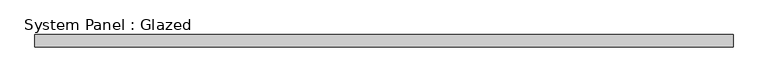
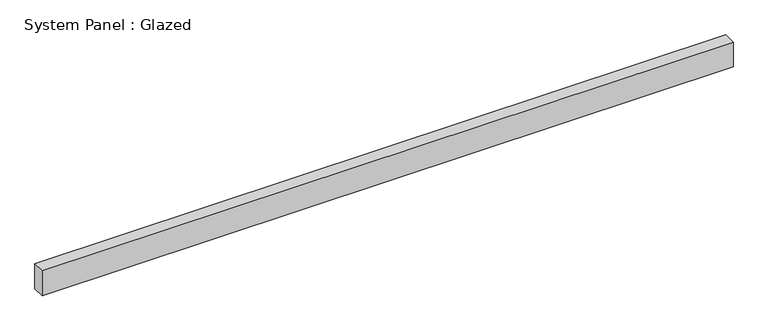
"""IFC4 building model written with IfcOpenShell, lengths in millimetres: plate geometry, System Panel : Glazed."""

from ifc_helpers import new_model, si_unit, origin, origin_with_axes, place, context, project, spatial, polyline, outline, extrude, source, transform, mapped, element, save


def system_panel_glazed_dde0d99a(model_context):
    return source(origin(), model_context, "Body", "SweptSolid", [
        extrude(outline(polyline([(704.8499999, 19.05), (-704.8499999, 19.05), (-704.8499999, 44.45), (704.8499999, 44.45), (704.8499999, 19.05)])), origin_with_axes(), (0.0, 0.0, 1.0), 53.5691055),
    ])


if __name__ == "__main__":
    model = new_model("IFC4")
    model_context = context("Model", 3, world=origin())
    ifc_project = project(units=[si_unit("LENGTHUNIT", "METRE", prefix="MILLI")], contexts=[model_context])
    site = spatial("IfcSite", under=ifc_project)
    building = spatial("IfcBuilding", under=site)
    placement = place(None, origin())
    system_panel_glazed_shape = system_panel_glazed_dde0d99a(model_context)
    element("IfcPlate", 1, ObjectType="System Panel : Glazed", at=placement, inside=building, context=model_context, shape_type="MappedRepresentation", body=[
        mapped(system_panel_glazed_shape, transform((0.0, 0.0, 0.0), x_axis=(1.0, 0.0, 0.0), y_axis=(0.0, 1.0, 0.0), z_axis=(0.0, 0.0, 1.0))),
    ])
    save(model, "model.ifc")

# Revit data of these elements
# Type "System Panel : Glazed"
#   Construction Type Id = "GSP4R"
#   Analytic Construction = "1/8 in Pilkington single glazing"
#   Visual Light Transmittance = 0.9
#   Solar Heat Gain Coefficient = 0.86
#   Heat Transfer Coefficient (U) = 1.18115 BTU/(h·ft²·°F)
#   Define Thermal Properties by = 1
# Element 1 (IfcPlate, "System Panel : Glazed")
#   Materials on its faces: "Glass"
# Materials
#   "Glass": class "Glass", colour RGB 0 128 192, transparency 0.75, Description = "Soda Lime Glass", Cost = 0
